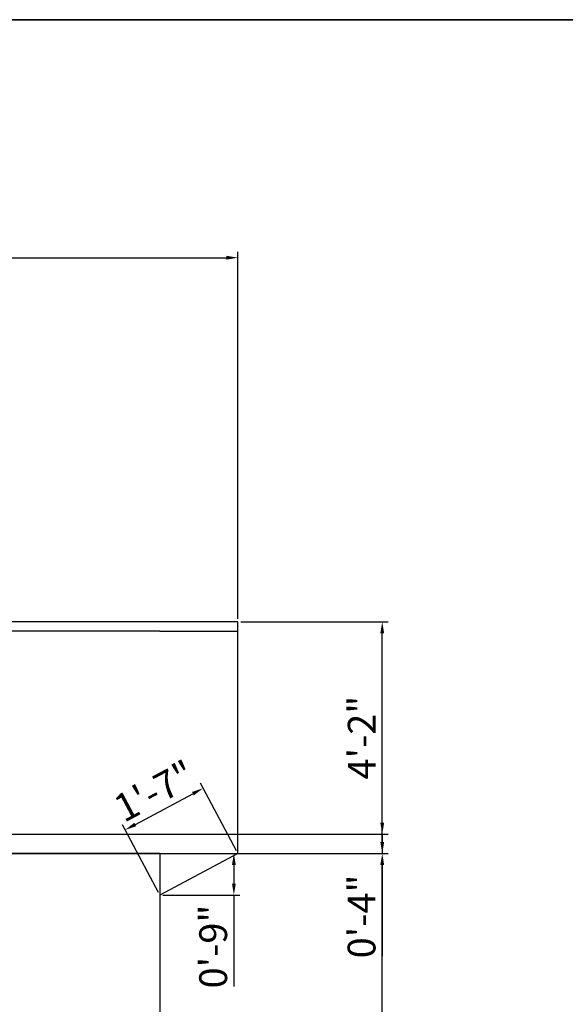
# Model space of a CAD drawing. Units: inches. Extents: x 2656 to 9931, y 1941 to 3068.
# Tile 44 of 46: x 2968 to 3086, y 2855 to 3068. Entities that reach past the tile are written whole.
import ezdxf

# ---------------------------------------------------------------- set-up
doc = ezdxf.new("R2010")
doc.units = ezdxf.units.IN
for name, color, linetype, lineweight in [('A-ANNO-DIMS', 2, 'Continuous', 18), ('A-ANNO-TTLB', 7, 'Continuous', 35), ('A-ELEV', 7, 'Continuous', 25)]:
    doc.layers.add(name, color=color, linetype=linetype, lineweight=lineweight)
doc.styles.get("Standard").update_dxf_attribs({"font": 'arial.ttf'})
doc.dimstyles.new('ISO-25', dxfattribs={"dimtxt": 6, "dimasz": 2.5, "dimexe": 1.25, "dimexo": 0.625, "dimtad": 1, "dimdec": 0, "dimlunit": 3, "dimtxsty": 'Standard', "dimcen": 2.5, "dimadec": 0, "dimazin": 0, "dimtfac": 1, "dimtdec": 0, "dimtmove": 0, "dimatfit": 3, "dimfxl": 1, "dimarcsym": 0})

# ---------------------------------------------------------------- blocks, each defined once
blk = doc.blocks.new('*D80')
at = {"layer": 'A-ANNO-DIMS', "color": 0, "lineweight": -2, "transparency": 16777216}
for p, q in [((3015.61, 2887.89), (3047.36, 2887.89)), ((3046.11, 2800.39), (3046.11, 2885.39)), ((2998.78, 2797.89), (3047.36, 2797.89))]:
    blk.add_line(p, q, dxfattribs=at)
at = {"layer": 'A-ANNO-DIMS', "color": 0, "transparency": 16777216}
for points in [[(3045.69, 2885.39), (3046.53, 2885.39), (3046.11, 2887.89)], [(3045.69, 2800.39), (3046.53, 2800.39), (3046.11, 2797.89)]]:
    blk.add_solid(points, dxfattribs=at)
at = {"layer": 'Defpoints', "color": 0, "transparency": 16777216}
for p in [(3014.98, 2887.89), (3046.11, 2887.89), (2998.16, 2797.89)]:
    blk.add_point(p, dxfattribs=at)
at = {"layer": 'A-ANNO-DIMS', "color": 0, "transparency": 16777216, "insert": (3042.42, 2842.89), "char_height": 6, "attachment_point": 5, "rotation": 90}
blk.add_mtext('7\'-6"', dxfattribs=at)
blk = doc.blocks.new('*D81')
at = {"layer": 'A-ANNO-DIMS', "color": 0, "lineweight": -2, "transparency": 16777216}
for p, q in [((3015.61, 2937.89), (3047.36, 2937.89)), ((3046.11, 2890.39), (3046.11, 2935.39)), ((3015.61, 2887.89), (3047.36, 2887.89))]:
    blk.add_line(p, q, dxfattribs=at)
at = {"layer": 'A-ANNO-DIMS', "color": 0, "transparency": 16777216}
for points in [[(3045.69, 2935.39), (3046.53, 2935.39), (3046.11, 2937.89)], [(3045.69, 2890.39), (3046.53, 2890.39), (3046.11, 2887.89)]]:
    blk.add_solid(points, dxfattribs=at)
at = {"layer": 'Defpoints', "color": 0, "transparency": 16777216}
for p in [(3014.98, 2937.89), (3046.11, 2937.89), (3014.98, 2887.89)]:
    blk.add_point(p, dxfattribs=at)
at = {"layer": 'A-ANNO-DIMS', "color": 0, "transparency": 16777216, "insert": (3042.47, 2912.89), "char_height": 6, "attachment_point": 5, "rotation": 90}
blk.add_mtext('4\'-2"', dxfattribs=at)
blk = doc.blocks.new('*D85')
at = {"layer": 'A-ANNO-DIMS', "color": 0, "lineweight": -2, "transparency": 16777216}
for p, q in [((2876.66, 3001.14), (2876.66, 3017.72)), ((3014.98, 2938.52), (3014.98, 3017.72)), ((2879.16, 3016.47), (3012.48, 3016.47))]:
    blk.add_line(p, q, dxfattribs=at)
at = {"layer": 'A-ANNO-DIMS', "color": 0, "transparency": 16777216}
for points in [[(2879.16, 3016.88), (2879.16, 3016.05), (2876.66, 3016.47)], [(3012.48, 3016.88), (3012.48, 3016.05), (3014.98, 3016.47)]]:
    blk.add_solid(points, dxfattribs=at)
at = {"layer": 'Defpoints', "color": 0, "transparency": 16777216}
for p in [(3014.98, 3016.47), (2876.66, 3000.52), (3014.98, 2937.89)]:
    blk.add_point(p, dxfattribs=at)
at = {"layer": 'A-ANNO-DIMS', "color": 0, "transparency": 16777216, "insert": (2945.82, 3020.19), "char_height": 6, "attachment_point": 5}
blk.add_mtext('11\'-6 1/2"', dxfattribs=at)
blk = doc.blocks.new('*D150')
at = {"layer": 'A-ANNO-DIMS', "color": 0, "lineweight": -2, "transparency": 16777216}
for p, q in [((3046.11, 2894.54), (3046.11, 2897.04)), ((2868.85, 2892.04), (3047.36, 2892.04)), ((3046.11, 2892.04), (3046.11, 2887.89)), ((2874.53, 2887.89), (3047.36, 2887.89)), ((3046.11, 2885.39), (3046.11, 2865.69))]:
    blk.add_line(p, q, dxfattribs=at)
at = {"layer": 'A-ANNO-DIMS', "color": 0, "transparency": 16777216}
for points in [[(3045.69, 2894.54), (3046.53, 2894.54), (3046.11, 2892.04)], [(3045.69, 2885.39), (3046.53, 2885.39), (3046.11, 2887.89)]]:
    blk.add_solid(points, dxfattribs=at)
at = {"layer": 'Defpoints', "color": 0, "transparency": 16777216}
for p in [(2868.23, 2892.04), (2873.91, 2887.89), (3046.11, 2887.89)]:
    blk.add_point(p, dxfattribs=at)
at = {"layer": 'A-ANNO-DIMS', "color": 0, "transparency": 16777216, "insert": (3042.42, 2874.29), "char_height": 6, "attachment_point": 5, "rotation": 90}
blk.add_mtext('0\'-4"', dxfattribs=at)
blk = doc.blocks.new('*D167')
at = {"layer": 'A-ANNO-DIMS', "color": 0, "lineweight": -2, "transparency": 16777216}
for p, q in [((3014.69, 2888.44), (3006.88, 2903.06)), ((2992.85, 2894.15), (3005.26, 2900.78)), ((2997.86, 2879.46), (2990.05, 2894.07))]:
    blk.add_line(p, q, dxfattribs=at)
at = {"layer": 'A-ANNO-DIMS', "color": 0, "transparency": 16777216}
for points in [[(3005.06, 2901.15), (3005.46, 2900.42), (3007.47, 2901.96)], [(2992.65, 2894.52), (2993.04, 2893.78), (2990.64, 2892.97)]]:
    blk.add_solid(points, dxfattribs=at)
at = {"layer": 'Defpoints', "color": 0, "transparency": 16777216}
for p in [(3007.47, 2901.96), (3014.98, 2887.89), (2998.16, 2878.9)]:
    blk.add_point(p, dxfattribs=at)
at = {"layer": 'A-ANNO-DIMS', "color": 0, "transparency": 16777216, "insert": (2997.34, 2900.67), "char_height": 6, "attachment_point": 5, "rotation": 28.115}
blk.add_mtext('1\'-7"', dxfattribs=at)
blk = doc.blocks.new('*D168')
at = {"layer": 'A-ANNO-DIMS', "color": 0, "lineweight": -2, "transparency": 16777216}
for p, q in [((2998.78, 2887.89), (3015.36, 2887.89)), ((3014.11, 2885.39), (3014.11, 2881.4)), ((2998.78, 2878.9), (3015.36, 2878.9)), ((3014.11, 2878.9), (3014.11, 2859.2))]:
    blk.add_line(p, q, dxfattribs=at)
at = {"layer": 'A-ANNO-DIMS', "color": 0, "transparency": 16777216}
for points in [[(3013.69, 2885.39), (3014.52, 2885.39), (3014.11, 2887.89)], [(3013.69, 2881.4), (3014.52, 2881.4), (3014.11, 2878.9)]]:
    blk.add_solid(points, dxfattribs=at)
at = {"layer": 'Defpoints', "color": 0, "transparency": 16777216}
for p in [(2998.16, 2887.89), (2998.16, 2878.9), (3014.11, 2878.9)]:
    blk.add_point(p, dxfattribs=at)
at = {"layer": 'A-ANNO-DIMS', "color": 0, "transparency": 16777216, "insert": (3010.42, 2867.8), "char_height": 6, "attachment_point": 5, "rotation": 90}
blk.add_mtext('0\'-9"', dxfattribs=at)

msp = doc.modelspace()

# ---------------------------------------------------------------- linework, layer by layer
at = {"layer": 'A-ANNO-TTLB'}
msp.add_lwpolyline([(2655.77, 3067.84), (3515.43, 3067.84), (3515.43, 1940.89), (2655.77, 1940.89)], close=True, dxfattribs=at)
at = {"layer": 'A-ELEV'}
for p, q in [((2998.16, 2937.89), (2876.66, 2937.89)), ((3014.98, 2937.89), (2998.16, 2937.89)), ((3014.98, 2887.89), (3014.98, 2937.89)), ((2998.16, 2935.89), (2935.96, 2935.89)), ((2998.16, 2935.89), (3014.98, 2935.89)), ((2998.16, 2887.89), (2743.16, 2887.89)), ((2998.16, 2887.89), (2998.16, 2797.89)), ((2998.16, 2887.89), (3014.98, 2887.89)), ((3014.98, 2887.89), (2998.16, 2878.9)), ((3014.98, 2887.89), (3014.98, 2887.89))]:
    msp.add_line(p, q, dxfattribs=at)

# ---------------------------------------------------------------- dimensions: what is measured, and where the dimension line sits
at = {"layer": 'A-ANNO-DIMS'}
dim = msp.add_linear_dim(base=(3014.98, 3016.47), p1=(2876.66, 3000.52), p2=(3014.98, 2937.89), dimstyle='ISO-25', override={"dimdec": 1, "dimlfac": 1, "dimrnd": 0, "dimzin": 1, "dimdsep": 46, "dimlunit": 4, "dimfrac": 2}, dxfattribs=at)
dim.commit()
dim.dimension.update_dxf_attribs({"geometry": '*D85', "text_midpoint": (2945.82, 3020.19)})
for base, p1, p2, angle, picture, middle in [((3046.11, 2937.89), (3014.98, 2887.89), (3014.98, 2937.89), 90, '*D81', (3042.47, 2912.89)), ((3007.47, 2901.96), (2998.16, 2878.9), (3014.98, 2887.89), 28.115, '*D167', (2997.34, 2900.67)), ((3046.11, 2887.8931), (2868.2256, 2892.0351), (2873.907, 2887.8931), 90, '*D150', (3042.4215, 2874.2933)), ((3046.11, 2887.89), (2998.16, 2797.89), (3014.98, 2887.89), 90, '*D80', (3042.42, 2842.89)), ((3014.11, 2878.9), (2998.16, 2887.89), (2998.16, 2878.9), 270, '*D168', (3010.42, 2867.8))]:
    dim = msp.add_linear_dim(base=base, p1=p1, p2=p2, angle=angle, dimstyle='ISO-25', override={"dimdec": 1, "dimlfac": 1, "dimrnd": 0, "dimzin": 1, "dimdsep": 46, "dimlunit": 4, "dimfrac": 2}, dxfattribs=at)
    dim.commit()
    dim.dimension.update_dxf_attribs({"geometry": picture, "text_midpoint": middle})

doc.saveas('drawing.dxf')
